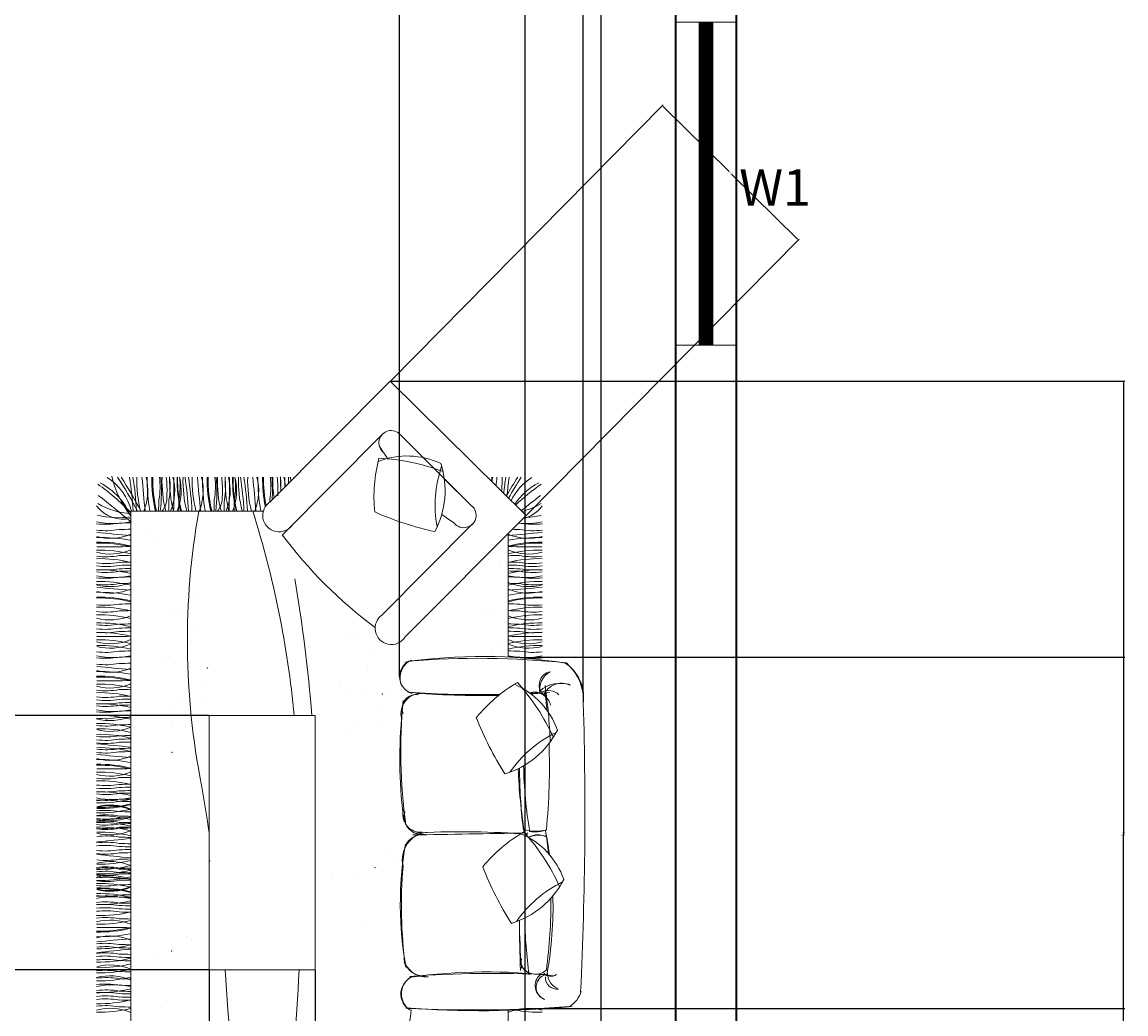
# Model space of a CAD drawing. Units: inches. Extents: x 318 to 927, y -1130 to 13.
# Tile 11 of 17: x 763 to 927, y -587 to -440. Entities that reach past the tile are written whole.
import ezdxf

# ---------------------------------------------------------------- set-up
doc = ezdxf.new("R2010")
doc.units = ezdxf.units.IN
doc.header["$MEASUREMENT"] = 0
for name, color, linetype, lineweight in [('A-ANNO-DIMS', 1, 'Continuous', 18), ('A-ANNO-IDEN', 1, 'Continuous', 13), ('A-FURN-RUGS', 50, 'Continuous', 9), ('A-GLAZ-PATT', 5, 'Continuous', 9), ('wall', 1, 'Continuous', 35), ('win', 5, 'Continuous', 18)]:
    doc.layers.add(name, color=color, linetype=linetype, lineweight=lineweight)
doc.layers.add('furniture', color=50, linetype='Continuous', lineweight=13, transparency=0.8)
doc.styles.get("Standard").update_dxf_attribs({"font": 'arial.ttf'})
doc.dimstyles.get("Standard").update_dxf_attribs({"dimtxt": 0.18, "dimasz": 0.18, "dimexe": 0.18, "dimexo": 0.0625, "dimgap": 0.09, "dimtad": 0, "dimtih": 1, "dimtoh": 1, "dimdec": 1, "dimzin": 0, "dimdsep": 46, "dimlunit": 4, "dimtxsty": 'Standard', "dimcen": 0.09, "dimadec": 0, "dimazin": 0, "dimtfac": 1, "dimtdec": 1, "dimtofl": 0, "dimtmove": 0, "dimatfit": 3, "dimfxl": 1, "dimtolj": 1, "dimtzin": 0, "dimarcsym": 0})

# ---------------------------------------------------------------- blocks, each defined once
blk = doc.blocks.new('WIN-48IN')
for p, q in [((0, 48), (9, 48)), ((3.5, 48), (3.5, 0)), ((5.5, 48), (5.5, 0)), ((0, 0), (9, 0))]:
    blk.add_line(p, q)
blk = doc.blocks.new('*D38')
at = {"layer": 'A-ANNO-DIMS', "color": 0, "lineweight": -2, "transparency": 16777216}
for p, q in [((817.59, -493.51), (926.57, -493.51)), ((926.39, -493.69), (926.39, -560.77)), ((926.39, -628.21), (926.39, -561.13)), ((817.59, -628.39), (926.57, -628.39))]:
    blk.add_line(p, q, dxfattribs=at)
at = {"layer": 'A-ANNO-DIMS', "color": 0, "transparency": 16777216}
for points in [[(926.36, -493.69), (926.42, -493.69), (926.39, -493.51)], [(926.36, -628.21), (926.42, -628.21), (926.39, -628.39)]]:
    blk.add_solid(points, dxfattribs=at)
at = {"layer": 'Defpoints', "color": 0, "transparency": 16777216}
for p in [(817.52, -493.51), (817.52, -628.39), (926.39, -628.39)]:
    blk.add_point(p, dxfattribs=at)
at = {"layer": 'A-ANNO-DIMS', "color": 0, "transparency": 16777216, "insert": (926.39, -560.95), "char_height": 0.18, "attachment_point": 5}
blk.add_mtext('\\A1;11\'-3"', dxfattribs=at)
blk = doc.blocks.new('*D40')
at = {"layer": 'A-ANNO-DIMS', "color": 0, "lineweight": -2, "transparency": 16777216}
for p, q in [((790.65, -580.99), (790.65, -1124.59)), ((806.39, -580.99), (806.39, -1124.59)), ((790.83, -1124.41), (797.99, -1124.41)), ((806.21, -1124.41), (799.05, -1124.41))]:
    blk.add_line(p, q, dxfattribs=at)
at = {"layer": 'A-ANNO-DIMS', "color": 0, "transparency": 16777216}
for points in [[(790.83, -1124.38), (790.83, -1124.44), (790.65, -1124.41)], [(806.21, -1124.38), (806.21, -1124.44), (806.39, -1124.41)]]:
    blk.add_solid(points, dxfattribs=at)
at = {"layer": 'Defpoints', "color": 0, "transparency": 16777216}
for p in [(790.65, -580.93), (806.39, -580.93), (806.39, -1124.41)]:
    blk.add_point(p, dxfattribs=at)
at = {"layer": 'A-ANNO-DIMS', "color": 0, "transparency": 16777216, "insert": (798.52, -1124.41), "char_height": 0.18, "attachment_point": 5}
blk.add_mtext('\\A1;1\'-3 1/2"', dxfattribs=at)
blk = doc.blocks.new('*D41')
at = {"layer": 'A-ANNO-DIMS', "color": 0, "lineweight": -2, "transparency": 16777216}
for p, q in [((790.59, -543.15), (331.21, -543.15)), ((331.39, -543.33), (331.39, -561.86)), ((331.39, -580.75), (331.39, -562.22)), ((790.59, -580.93), (331.21, -580.93))]:
    blk.add_line(p, q, dxfattribs=at)
at = {"layer": 'A-ANNO-DIMS', "color": 0, "transparency": 16777216}
for points in [[(331.36, -543.33), (331.42, -543.33), (331.39, -543.15)], [(331.36, -580.75), (331.42, -580.75), (331.39, -580.93)]]:
    blk.add_solid(points, dxfattribs=at)
at = {"layer": 'Defpoints', "color": 0, "transparency": 16777216}
for p in [(790.65, -543.15), (331.39, -580.93), (790.65, -580.93)]:
    blk.add_point(p, dxfattribs=at)
at = {"layer": 'A-ANNO-DIMS', "color": 0, "transparency": 16777216, "insert": (331.39, -562.04), "char_height": 0.18, "attachment_point": 5}
blk.add_mtext('\\A1;3\'-2"', dxfattribs=at)
blk = doc.blocks.new('*D42')
at = {"layer": 'A-ANNO-DIMS', "color": 0, "lineweight": -2, "transparency": 16777216}
for p, q in [((838.899969, -534.470376), (926.574248, -534.470376)), ((926.394248, -534.650376), (926.394248, -560.388084)), ((926.394248, -586.485792), (926.394248, -560.748084)), ((838.877744, -586.665792), (926.574248, -586.665792))]:
    blk.add_line(p, q, dxfattribs=at)
at = {"layer": 'A-ANNO-DIMS', "color": 0, "transparency": 16777216}
for points in [[(926.364248, -534.650376), (926.424248, -534.650376), (926.394248, -534.470376)], [(926.364248, -586.485792), (926.424248, -586.485792), (926.394248, -586.665792)]]:
    blk.add_solid(points, dxfattribs=at)
at = {"layer": 'Defpoints', "color": 0, "transparency": 16777216}
for p in [(838.837469, -534.470376), (838.815244, -586.665792), (926.394248, -586.665792)]:
    blk.add_point(p, dxfattribs=at)
at = {"layer": 'A-ANNO-DIMS', "color": 0, "transparency": 16777216, "insert": (926.394248, -560.568084), "char_height": 0.18, "attachment_point": 5}
blk.add_mtext('\\A1;4\'-4"', dxfattribs=at)
blk = doc.blocks.new('*D43')
at = {"layer": 'A-ANNO-DIMS', "color": 0, "lineweight": -2, "transparency": 16777216}
for p, q in [((818.92, -537.33), (818.92, -25.23)), ((819.1, -25.41), (832.2, -25.41)), ((845.97, -25.41), (832.87, -25.41)), ((846.15, -539.79), (846.15, -25.23))]:
    blk.add_line(p, q, dxfattribs=at)
at = {"layer": 'A-ANNO-DIMS', "color": 0, "transparency": 16777216}
for points in [[(819.1, -25.38), (819.1, -25.44), (818.92, -25.41)], [(845.97, -25.38), (845.97, -25.44), (846.15, -25.41)]]:
    blk.add_solid(points, dxfattribs=at)
at = {"layer": 'Defpoints', "color": 0, "transparency": 16777216}
for p in [(846.15, -25.41), (818.92, -537.39), (846.15, -539.86)]:
    blk.add_point(p, dxfattribs=at)
at = {"layer": 'A-ANNO-DIMS', "color": 0, "transparency": 16777216, "insert": (832.53, -25.41), "char_height": 0.18, "attachment_point": 5}
blk.add_mtext('\\A1;2\'-3"', dxfattribs=at)
blk = doc.blocks.new('*D44')
at = {"layer": 'A-ANNO-DIMS', "color": 0, "lineweight": -2, "transparency": 16777216}
for p, q in [((817.57, -493.47), (858.05, -452.47)), ((858.05, -452.72), (867.82, -462.37)), ((877.96, -472.38), (868.19, -462.74)), ((837.73, -513.38), (878.22, -472.38))]:
    blk.add_line(p, q, dxfattribs=at)
at = {"layer": 'A-ANNO-DIMS', "color": 0, "transparency": 16777216}
for points in [[(858.07, -452.7), (858.03, -452.74), (857.92, -452.6)], [(877.98, -472.36), (877.94, -472.41), (878.09, -472.51)]]:
    blk.add_solid(points, dxfattribs=at)
at = {"layer": 'Defpoints', "color": 0, "transparency": 16777216}
for p in [(878.09, -472.51), (817.52, -493.51), (837.69, -513.42)]:
    blk.add_point(p, dxfattribs=at)
at = {"layer": 'A-ANNO-DIMS', "color": 0, "transparency": 16777216, "insert": (868.01, -462.55), "char_height": 0.18, "attachment_point": 5}
blk.add_mtext('\\A1;2\'-4 1/2"', dxfattribs=at)
blk = doc.blocks.new('*D53')
at = {"layer": 'A-ANNO-DIMS', "color": 0, "lineweight": -2, "transparency": 16777216}
for p, q in [((837.57, -839.31), (837.57, -25.23)), ((837.75, -25.41), (842.6, -25.41)), ((848.66, -25.41), (843.82, -25.41)), ((848.84, -838.59), (848.84, -25.23))]:
    blk.add_line(p, q, dxfattribs=at)
at = {"layer": 'A-ANNO-DIMS', "color": 0, "transparency": 16777216}
for points in [[(837.75, -25.38), (837.75, -25.44), (837.57, -25.41)], [(848.66, -25.38), (848.66, -25.44), (848.84, -25.41)]]:
    blk.add_solid(points, dxfattribs=at)
at = {"layer": 'Defpoints', "color": 0, "transparency": 16777216}
for p in [(848.84, -25.41), (848.84, -838.66), (837.57, -839.37)]:
    blk.add_point(p, dxfattribs=at)
at = {"layer": 'A-ANNO-DIMS', "color": 0, "transparency": 16777216, "insert": (843.21, -25.41), "char_height": 0.18, "attachment_point": 5}
blk.add_mtext('\\A1;0\'-11 1/2"', dxfattribs=at)

msp = doc.modelspace()

# ---------------------------------------------------------------- hatches: boundary and pattern name
at = {"layer": 'A-GLAZ-PATT'}
h = msp.add_hatch(dxfattribs=at)
h.set_pattern_fill('ANSI31', color=256)
h.paths.add_polyline_path([(865.39, -312.52), (863.39, -312.52), (863.39, -348.52), (865.39, -348.52)])
h.paths.add_polyline_path([(865.39, -440.16), (863.39, -440.16), (863.39, -488.16), (865.39, -488.16)])
h.paths.add_polyline_path([(865.39, -635.51), (863.39, -635.51), (863.39, -683.51), (865.39, -683.51)])
h.paths.add_polyline_path([(865.39, -778.6), (863.39, -778.6), (863.39, -814.6), (865.39, -814.6)])
h.paths.add_polyline_path([(865.39, -834.21), (863.39, -834.21), (863.39, -870.21), (865.39, -870.21)])

# ---------------------------------------------------------------- linework, layer by layer
at = {"layer": 'A-FURN-RUGS'}
for p, q in [((786.52, -509.62), (786.52, -509.62)), ((786.56, -510.1), (786.56, -510.1)), ((794.75, -509.62), (794.75, -509.62)), ((794.79, -510.1), (794.79, -510.1)), ((779, -612.91), (779, -512.79)), ((779, -512.79), (798.69, -512.79)), ((777.42, -514.38), (777.42, -514.38)), ((777.42, -514.38), (777.42, -514.38)), ((777.42, -514.38), (777.42, -514.38)), ((836.61, -514.38), (836.61, -514.38)), ((836.61, -514.38), (836.61, -514.38)), ((836.61, -514.38), (836.61, -514.38)), ((777.71, -515.6), (777.71, -515.6)), ((777.71, -515.6), (777.71, -515.6)), ((777.71, -515.6), (777.71, -515.6)), ((781.73, -515.62), (781.73, -515.62)), ((835.03, -516.09), (835.03, -534.47)), ((836.32, -515.6), (836.32, -515.6)), ((836.32, -515.6), (836.32, -515.6)), ((836.32, -515.6), (836.32, -515.6)), ((782.8, -517.13), (782.8, -517.13)), ((835.56, -518.24), (835.56, -518.24)), ((835.56, -518.24), (835.56, -518.24)), ((832.07, -519.93), (832.07, -519.93)), ((833.84, -520.06), (833.84, -520.06)), ((835.98, -522.53), (835.98, -522.53)), ((835.36, -524.31), (835.36, -524.31)), ((788.26, -525.92), (788.26, -525.92)), ((788.26, -525.92), (788.26, -525.92)), ((784.78, -527.61), (784.78, -527.61)), ((831.36, -527.46), (831.36, -527.46)), ((832.88, -527.58), (832.88, -527.58)), ((779, -528.62), (779, -612.91)), ((786.55, -527.74), (786.55, -527.74)), ((835.06, -528.35), (835.06, -528.35)), ((838, -528.06), (838, -528.06)), ((788.69, -530.21), (788.69, -530.21)), ((814.27, -529.76), (814.27, -529.76)), ((814.27, -529.76), (814.27, -529.76)), ((837.28, -530.85), (837.28, -530.85)), ((788.06, -531.99), (788.06, -531.99)), ((810.79, -531.45), (810.79, -531.45)), ((812.56, -531.58), (812.56, -531.58)), ((814.7, -534.05), (814.7, -534.05)), ((832.56, -534.17), (832.56, -534.17)), ((833.28, -532.67), (833.28, -532.67)), ((837.48, -533.22), (837.48, -533.22)), ((784.07, -535.14), (784.07, -535.14)), ((785.59, -535.26), (785.59, -535.26)), ((790.71, -535.74), (790.71, -535.74)), ((787.77, -536.03), (787.77, -536.03)), ((814.08, -535.83), (814.08, -535.83)), ((789.98, -538.53), (789.98, -538.53)), ((810.08, -538.98), (810.08, -538.98)), ((785.99, -540.35), (785.99, -540.35)), ((811.6, -539.1), (811.6, -539.1)), ((813.78, -539.87), (813.78, -539.87)), ((816.72, -539.59), (816.72, -539.59)), ((785.26, -541.85), (785.26, -541.85)), ((790.19, -540.91), (790.19, -540.91)), ((816, -542.37), (816, -542.37)), ((785.23, -543.92), (785.23, -543.92)), ((812, -544.19), (812, -544.19)), ((816.2, -544.75), (816.2, -544.75)), ((811.28, -545.69), (811.28, -545.69)), ((777.42, -555.75), (777.42, -555.75)), ((777.42, -555.86), (777.42, -555.86)), ((777.42, -559.27), (777.42, -559.27)), ((817.37, -563.55), (817.37, -563.55)), ((817.37, -563.55), (817.37, -563.55)), ((815.49, -565.31), (815.49, -565.31)), ((818.2, -564.09), (818.2, -564.09)), ((818.2, -564.09), (818.2, -564.09)), ((777.42, -566.43), (777.42, -566.43)), ((809.01, -566.45), (809.01, -566.45)), ((812.75, -566.4), (812.75, -566.4)), ((777.42, -569.84), (777.42, -569.84)), ((777.42, -569.95), (777.42, -569.95)), ((813.75, -573.98), (813.75, -573.98)), ((787.23, -575.93), (787.23, -575.93)), ((787.23, -575.93), (787.23, -575.93)), ((788.05, -576.48), (788.05, -576.48)), ((788.05, -576.48), (788.05, -576.48)), ((785.34, -577.7), (785.34, -577.7)), ((778.87, -578.84), (778.87, -578.84)), ((782.6, -578.78), (782.6, -578.78)), ((783.6, -586.37), (783.6, -586.37)), ((835.03, -586.93), (835.03, -589.47))]:
    msp.add_line(p, q, dxfattribs=at)
for centre, radius, start, end in [((771.07, -514.79), 8.28, 13.9935, 57.7288), ((790.74, -504.28), 14.92, 192.9523, 218.0769), ((729.8, -538.65), 56.46, 27.2669, 33.1781), ((730.31, -538.64), 56.46, 27.2669, 33.1781), ((724.61, -515.98), 54.84, 3.3644, 8.6229), ((725.12, -515.97), 54.84, 3.3644, 8.6229), ((799.08, -508.19), 19.18, 178.6331, 193.8573), ((557.89, -530.4), 223.93, 4.5146, 5.8017), ((773.68, -509.76), 7.87, 337.3098, 14.8613), ((806.9, -508.17), 25.47, 179.0195, 190.4039), ((801.3, -508.2), 19.18, 178.6331, 193.8573), ((801.45, -508.2), 19.18, 178.6331, 193.8573), ((771.97, -509.1), 11.39, 349.9349, 6.8829), ((757.66, -509.77), 25.91, 353.3702, 4.5064), ((802.82, -508.19), 19.18, 178.6331, 193.8573), ((766.64, -509.72), 17.75, 357.4435, 6.4413), ((773.46, -509.1), 11.39, 349.9349, 6.8829), ((803.95, -508.18), 19.18, 178.6331, 193.8573), ((777.66, -509.75), 7.87, 337.3098, 14.8613), ((621.19, -508.91), 164.23, 358.628, 0.3934), ((778.63, -509.76), 7.87, 337.3098, 14.8613), ((805.08, -508.2), 19.18, 178.6331, 193.8573), ((805.14, -508.19), 19.18, 178.6331, 193.8573), ((774.95, -509.11), 11.39, 349.9349, 6.8829), ((805.94, -508.2), 19.18, 178.6331, 193.8573), ((732.84, -515.98), 54.84, 3.3644, 8.6229), ((733.35, -515.97), 54.84, 3.3644, 8.6229), ((807.31, -508.19), 19.18, 178.6331, 193.8573), ((566.11, -530.4), 223.93, 4.5146, 5.8017), ((781.9, -509.76), 7.87, 337.3098, 14.8613), ((815.12, -508.17), 25.47, 179.0195, 190.4039), ((809.53, -508.2), 19.18, 178.6331, 193.8573), ((809.67, -508.2), 19.18, 178.6331, 193.8573), ((780.19, -509.1), 11.39, 349.9349, 6.8829), ((765.88, -509.77), 25.91, 353.3702, 4.5064), ((811.04, -508.19), 19.18, 178.6331, 193.8573), ((774.87, -509.72), 17.75, 357.4435, 6.4413), ((781.69, -509.1), 11.39, 349.9349, 6.8829), ((812.18, -508.18), 19.18, 178.6331, 193.8573), ((785.89, -509.75), 7.87, 337.3098, 14.8613), ((629.42, -508.91), 164.23, 358.628, 0.3934), ((786.85, -509.76), 7.87, 337.3098, 14.8613), ((813.3, -508.2), 19.18, 178.6331, 193.8573), ((813.37, -508.19), 19.18, 178.6331, 193.8573), ((783.17, -509.11), 11.39, 349.9349, 6.8829), ((814.16, -508.2), 19.18, 178.6331, 193.8573), ((741.07, -515.98), 54.84, 3.3644, 8.6229), ((741.58, -515.97), 54.84, 3.3644, 8.6229), ((815.54, -508.19), 19.18, 178.6331, 193.8573), ((574.34, -530.4), 223.93, 4.5146, 5.8017), ((790.13, -509.76), 7.87, 337.3098, 14.8613), ((823.36, -508.17), 25.47, 179.0195, 190.4039), ((817.76, -508.2), 19.18, 178.6331, 191.8302), ((817.9, -508.2), 19.18, 178.6331, 191.3519), ((788.42, -509.1), 11.39, 349.9349, 6.8829), ((774.12, -509.77), 25.91, 356.9677, 4.5064), ((819.27, -508.19), 19.18, 178.6331, 187.9798), ((783.1, -509.72), 17.75, 357.4435, 6.4413), ((820.41, -508.18), 19.18, 178.6331, 184.9238), ((789.92, -509.1), 11.39, 356.2453, 6.8829), ((794.12, -509.75), 7.87, 4.2757, 14.8613), ((637.65, -508.91), 164.23, 359.8849, 0.3934), ((821.6, -508.19), 19.18, 178.6331, 181.5238), ((795.08, -509.76), 7.87, 10.6592, 14.8613), ((791.41, -509.11), 11.39, 3.8173, 6.8829), ((822.39, -508.2), 19.18, 178.6331, 179.1046), ((807.13, -508.17), 25.47, 359.4753, 0.9805), ((840.36, -509.76), 7.87, 165.1387, 170.0752), ((1056.15, -530.4), 223.93, 174.1983, 174.5236), ((814.95, -508.19), 19.18, 355.0538, 1.3669), ((888.91, -515.97), 54.84, 171.3771, 173.9203), ((883.72, -538.64), 56.46, 146.8219, 150.1356), ((889.42, -515.98), 54.84, 171.3771, 174.3888), ((884.23, -538.65), 56.46, 146.8219, 150.5026), ((842.96, -514.79), 8.28, 122.2712, 154.6274), ((754.54, -536.39), 33.84, 43.716, 54.6847), ((770.01, -517.21), 9.7, 22.1181, 62.6967), ((844.02, -517.21), 9.7, 117.3033, 145.7016), ((859.49, -536.39), 33.84, 125.3153, 133.6457), ((679.49, -633.67), 155.39, 50.1568, 52.4559), ((910.14, -515.1), 127.02, 178.1891, 178.9775), ((780.95, -510.71), 3.43, 321.6564, 3.1744), ((911.64, -515.1), 127.02, 178.1891, 178.9775), ((913.12, -515.11), 127.02, 178.1891, 178.9775), ((918.36, -515.1), 127.02, 178.1891, 178.9775), ((789.17, -510.71), 3.43, 321.6564, 3.1744), ((919.86, -515.1), 127.02, 178.1891, 178.9775), ((921.35, -515.11), 127.02, 178.1891, 178.9775), ((926.6, -515.1), 127.02, 178.1891, 178.3576), ((934.54, -633.67), 155.39, 127.5441, 128.8901), ((777.91, -509.12), 4.9, 215.9057, 282.8054), ((779.85, -501.71), 11.5, 240.135, 265.7243), ((897.54, -532.05), 110.13, 169.9275, 191.2246), ((656.23, -557.16), 147.71, 5.4421, 17.4799), ((834.18, -501.71), 11.5, 284.6792, 299.865), ((836.12, -509.12), 4.9, 282.9777, 324.0943), ((776.42, -501.87), 12.76, 258.7545, 281.5888), ((777.27, -499.93), 13.84, 256.7215, 277.1491), ((837.61, -501.87), 12.76, 265.1756, 281.2455), ((836.76, -499.93), 13.84, 272.5322, 283.2785), ((775.3, -503.36), 11.39, 263.1171, 280.0651), ((775.29, -504.31), 11.39, 263.1171, 280.0651), ((796.6, -293.17), 223.93, 264.1983, 265.4854), ((781.3, -642.48), 127.02, 91.0225, 91.8109), ((781.3, -641.53), 127.02, 91.0225, 91.8109), ((817.43, -293.17), 223.93, 274.5146, 275.8017), ((832.73, -642.48), 127.02, 88.1891, 88.6709), ((838.74, -503.36), 11.39, 259.9349, 276.8829), ((838.74, -504.31), 11.39, 259.9349, 276.8829), ((774.37, -542.18), 25.47, 79.5961, 90.9805), ((774.4, -536.59), 19.18, 76.1427, 91.3669), ((774.4, -536.73), 19.18, 76.1427, 91.3669), ((775.97, -508.96), 7.87, 255.1387, 292.6902), ((838.07, -508.96), 7.87, 247.3098, 284.8613), ((839.63, -536.59), 19.18, 88.6331, 103.8573), ((839.63, -536.73), 19.18, 88.6331, 103.8573), ((839.66, -542.18), 25.47, 89.0195, 100.4039), ((775.96, -511.3), 7.87, 255.1387, 292.6902), ((774.4, -537.76), 19.18, 76.1427, 91.3669), ((775.3, -508.18), 11.39, 263.1171, 280.0651), ((775.11, -353.87), 164.23, 269.6066, 271.372), ((781.31, -646.35), 127.02, 91.0225, 91.8109), ((838.92, -353.87), 164.23, 268.628, 270.3934), ((832.72, -646.35), 127.02, 88.1891, 88.9775), ((838.07, -511.3), 7.87, 247.3098, 284.8613), ((839.63, -537.76), 19.18, 88.6331, 103.8573), ((838.73, -508.18), 11.39, 259.9349, 276.8829), ((774.4, -539.03), 19.18, 76.1427, 91.3669), ((775.3, -509.18), 11.39, 263.1171, 280.0651), ((775.3, -509.63), 11.39, 263.1171, 280.0651), ((781.31, -647.36), 127.02, 91.0225, 91.8109), ((781.3, -647.81), 127.02, 91.0225, 91.8109), ((832.73, -647.36), 127.02, 88.1891, 88.9775), ((832.73, -647.81), 127.02, 88.1891, 88.9775), ((839.63, -539.03), 19.18, 88.6331, 103.8573), ((838.73, -509.18), 11.39, 259.9349, 276.8829), ((838.73, -509.63), 11.39, 259.9349, 276.8829), ((775.3, -510.14), 11.39, 263.1171, 280.0651), ((774.39, -540.68), 19.18, 76.1427, 91.3669), ((775.3, -510.51), 11.39, 263.1171, 280.0651), ((775.3, -511.38), 11.39, 263.1171, 280.0651), ((776.42, -509.9), 12.76, 258.7545, 281.5888), ((781.3, -648.31), 127.02, 91.0225, 91.8109), ((781.3, -648.68), 127.02, 91.0225, 91.8109), ((781.3, -649.56), 127.02, 91.0225, 91.8109), ((832.73, -648.31), 127.02, 88.1891, 88.9775), ((832.73, -648.68), 127.02, 88.1891, 88.9775), ((832.73, -649.56), 127.02, 88.1891, 88.9775), ((839.64, -540.68), 19.18, 88.6331, 103.8573), ((837.61, -509.9), 12.76, 258.4112, 281.2455), ((838.73, -510.14), 11.39, 259.9349, 276.8829), ((838.73, -510.51), 11.39, 259.9349, 276.8829), ((838.74, -511.38), 11.39, 259.9349, 276.8829), ((774.39, -542.42), 19.18, 76.1427, 91.3669), ((775.95, -516.13), 7.87, 255.1387, 292.6902), ((775.29, -512.34), 11.39, 263.1171, 280.0651), ((796.6, -301.31), 223.93, 264.1983, 265.4854), ((781.3, -650.51), 127.02, 91.0225, 91.8109), ((577.78, -561.59), 228.87, 4.6196, 9.7513), ((832.73, -650.51), 127.02, 88.1891, 88.9775), ((839.64, -542.42), 19.18, 88.6331, 103.8573), ((838.08, -516.13), 7.87, 247.3098, 284.8613), ((817.43, -301.31), 223.93, 274.5146, 275.8017), ((838.74, -512.34), 11.39, 259.9349, 276.8829), ((774.37, -550.32), 25.47, 79.5961, 90.9805), ((774.4, -544.73), 19.18, 76.1427, 91.3669), ((774.4, -544.87), 19.18, 76.1427, 91.3669), ((775.97, -517.1), 7.87, 255.1387, 292.6902), ((838.07, -517.1), 7.87, 247.3098, 284.8613), ((839.63, -544.73), 19.18, 88.6331, 103.8573), ((839.63, -544.87), 19.18, 88.6331, 103.8573), ((839.66, -550.32), 25.47, 89.0195, 100.4039), ((775.3, -515.39), 11.39, 263.1171, 280.0651), ((774.4, -546.24), 19.18, 76.1427, 91.3669), ((775.3, -516.4), 11.39, 263.1171, 280.0651), ((781.31, -653.56), 127.02, 91.0225, 91.8109), ((781.31, -654.57), 127.02, 91.0225, 91.8109), ((832.72, -653.56), 127.02, 88.1891, 88.9775), ((832.73, -654.57), 127.02, 88.1891, 88.9775), ((839.63, -546.24), 19.18, 88.6331, 103.8573), ((838.73, -515.39), 11.39, 259.9349, 276.8829), ((838.73, -516.4), 11.39, 259.9349, 276.8829), ((774.39, -547.37), 19.18, 76.1427, 91.3669), ((775.95, -521.08), 7.87, 255.1387, 292.6902), ((839.64, -547.37), 19.18, 88.6331, 103.8573), ((838.08, -521.08), 7.87, 247.3098, 284.8613), ((774.39, -548.57), 19.18, 76.1427, 91.3669), ((775.3, -519.46), 11.39, 263.1171, 280.0651), ((774.39, -550), 19.18, 76.1427, 91.3669), ((775.31, -518.37), 11.39, 263.1171, 280.0651), ((775.3, -518.96), 11.39, 263.1171, 280.0651), ((781.3, -657.13), 127.02, 91.0225, 91.8109), ((781.3, -657.63), 127.02, 91.0225, 91.8109), ((781.31, -656.54), 127.02, 91.0225, 91.8109), ((832.72, -656.54), 127.02, 88.1891, 88.9775), ((832.73, -657.13), 127.02, 88.1891, 88.9775), ((832.73, -657.63), 127.02, 88.1891, 88.9775), ((839.64, -550), 19.18, 88.6331, 103.8573), ((839.64, -548.57), 19.18, 88.6331, 103.8573), ((838.72, -518.37), 11.39, 259.9349, 276.8829), ((838.73, -518.96), 11.39, 259.9349, 276.8829), ((838.73, -519.46), 11.39, 259.9349, 276.8829), ((775.96, -524.62), 7.87, 255.1387, 292.6902), ((774.4, -551.07), 19.18, 76.1427, 91.3669), ((775.97, -525.28), 7.87, 255.1387, 292.6902), ((775.11, -367.19), 164.23, 269.6066, 271.372), ((838.92, -367.19), 164.23, 268.628, 270.3934), ((838.06, -525.28), 7.87, 247.3098, 284.8613), ((838.07, -524.62), 7.87, 247.3098, 284.8613), ((839.63, -551.07), 19.18, 88.6331, 103.8573), ((775.3, -522.38), 11.39, 263.1171, 280.0651), ((774.41, -551.93), 19.18, 76.1427, 91.3669), ((781.3, -660.55), 127.02, 91.0225, 91.8109), ((832.73, -660.55), 127.02, 88.1891, 88.9775), ((839.62, -551.93), 19.18, 88.6331, 103.8573), ((838.73, -522.38), 11.39, 259.9349, 276.8829), ((775.3, -523.26), 11.39, 263.1171, 280.0651), ((775.29, -524.21), 11.39, 263.1171, 280.0651), ((776.42, -521.77), 12.76, 258.7545, 281.5888), ((781.3, -662.38), 127.02, 91.0225, 91.8109), ((781.3, -661.43), 127.02, 91.0225, 91.8109), ((832.73, -661.43), 127.02, 88.1891, 88.9775), ((837.61, -521.77), 12.76, 258.4112, 281.2455), ((838.74, -523.26), 11.39, 259.9349, 276.8829), ((774.37, -562.08), 25.47, 79.5961, 90.9805), ((774.4, -556.49), 19.18, 76.1427, 91.3669), ((774.4, -556.63), 19.18, 76.1427, 91.3669), ((775.97, -528.86), 7.87, 255.1387, 292.6902), ((796.6, -313.07), 223.93, 264.1983, 265.4854), ((775.96, -531.2), 7.87, 255.1387, 292.6902), ((774.4, -557.66), 19.18, 76.1427, 91.3669), ((775.11, -373.77), 164.23, 269.6066, 271.372), ((775.3, -528.08), 11.39, 263.1171, 280.0651), ((774.4, -558.93), 19.18, 76.1427, 91.3669), ((775.3, -529.08), 11.39, 263.1171, 280.0651), ((781.31, -666.25), 127.02, 91.0225, 91.8109), ((781.31, -667.25), 127.02, 91.0225, 91.8109), ((781.3, -667.71), 127.02, 91.0225, 91.8109), ((775.3, -530.04), 11.39, 263.1171, 280.0651), ((774.39, -560.58), 19.18, 76.1427, 91.3669), ((775.3, -530.41), 11.39, 263.1171, 280.0651), ((775.3, -529.53), 11.39, 263.1171, 280.0651), ((776.42, -529.8), 12.76, 258.7545, 281.5888), ((781.3, -668.21), 127.02, 91.0225, 91.8109), ((781.3, -668.58), 127.02, 91.0225, 91.8109), ((775.3, -531.28), 11.39, 263.1171, 280.0651), ((774.39, -562.32), 19.18, 76.1427, 91.3669), ((775.95, -536.03), 7.87, 255.1387, 292.6902), ((775.29, -532.23), 11.39, 263.1171, 280.0651), ((781.3, -670.41), 127.02, 91.0225, 91.8109), ((781.3, -669.45), 127.02, 91.0225, 91.8109), ((774.39, -563.51), 19.18, 76.1427, 91.3669), ((775.31, -533.32), 11.39, 263.1171, 280.0651), ((775.97, -537.63), 7.87, 255.1387, 292.6902), ((774.41, -564.28), 19.18, 76.1427, 91.3669), ((781.31, -671.49), 127.02, 91.0225, 91.8109), ((775.29, -535.91), 11.39, 263.1171, 280.0651), ((775.31, -535.45), 11.39, 263.1171, 280.0651), ((774.4, -565.12), 19.18, 76.1427, 91.3669), ((775.31, -534.94), 11.39, 263.1171, 280.0651), ((781.3, -674.08), 127.02, 91.0225, 91.8109), ((781.31, -673.12), 127.02, 91.0225, 91.8109), ((781.31, -673.62), 127.02, 91.0225, 91.8109), ((774.41, -567.1), 19.18, 76.1427, 91.3669), ((775.31, -537.33), 11.39, 263.1171, 280.0651), ((734.62, -971.38), 425.85, 84.0165, 84.6992), ((775.32, -536.84), 11.39, 263.1171, 280.0651), ((781.32, -675.5), 127.02, 91.0225, 91.8109), ((781.33, -675.01), 127.02, 91.0225, 91.8109), ((774.37, -575.16), 25.47, 79.5961, 90.9805), ((774.4, -569.57), 19.18, 76.1427, 91.3669), ((774.4, -569.71), 19.18, 76.1427, 91.3669), ((775.97, -541.94), 7.87, 255.1387, 292.6902), ((796.6, -326.15), 223.93, 264.1983, 265.4854), ((775.96, -544.29), 7.87, 255.1387, 292.6902), ((774.4, -570.74), 19.18, 76.1427, 91.3669), ((775.11, -386.85), 164.23, 269.6066, 271.372), ((775.3, -541.16), 11.39, 263.1171, 280.0651), ((774.4, -572.01), 19.18, 76.1427, 91.3669), ((775.3, -542.16), 11.39, 263.1171, 280.0651), ((775.3, -542.62), 11.39, 263.1171, 280.0651), ((781.31, -679.33), 127.02, 91.0225, 91.8109), ((781.31, -680.34), 127.02, 91.0225, 91.8109), ((781.3, -680.79), 127.02, 91.0225, 91.8109), ((578.83, -590.81), 213.96, 8.119, 10.0442), ((775.3, -543.12), 11.39, 263.1171, 280.0651), ((774.39, -573.66), 19.18, 76.1427, 91.3669), ((775.3, -543.49), 11.39, 263.1171, 280.0651), ((776.42, -542.88), 12.76, 258.7545, 281.5888), ((781.3, -681.29), 127.02, 91.0225, 91.8109), ((781.3, -681.66), 127.02, 91.0225, 91.8109), ((775.3, -544.36), 11.39, 263.1171, 280.0651), ((774.39, -538.43), 19.18, 268.6331, 283.8573), ((774.4, -536.93), 19.18, 268.6331, 283.8573), ((775.31, -567.11), 11.39, 79.9349, 96.8829), ((774.41, -537.65), 19.18, 268.6331, 283.8573), ((774.41, -537.77), 19.18, 268.6331, 283.8573), ((775.97, -564.3), 7.87, 67.3098, 104.8613), ((775.97, -564.41), 7.87, 67.3098, 104.8613), ((781.3, -682.54), 127.02, 91.0225, 91.8109), ((781.31, -428.93), 127.02, 268.1891, 268.9775), ((774.39, -577.22), 19.18, 76.1427, 91.3669), ((775.95, -550.93), 7.87, 255.1387, 292.6902), ((775.29, -547.14), 11.39, 263.1171, 280.0651), ((775.31, -568.62), 11.39, 79.9349, 96.8829), ((775.32, -569.29), 11.39, 79.9349, 96.8829), ((734.62, -134.75), 425.85, 275.3008, 275.9835), ((781.3, -685.31), 127.02, 91.0225, 91.8109), ((781.31, -430.45), 127.02, 268.1891, 268.9775), ((781.33, -431.12), 127.02, 268.1891, 268.9775), ((775.29, -570.23), 11.39, 79.9349, 96.8829), ((774.39, -578.88), 19.18, 76.1427, 91.3669), ((775.31, -548.53), 11.39, 263.1171, 280.0651), ((775.31, -548.68), 11.39, 263.1171, 280.0651), ((774.4, -578.2), 19.18, 76.1427, 91.3669), ((775.31, -548.03), 11.39, 263.1171, 280.0651), ((775.97, -553), 7.87, 255.1387, 292.6902), ((781.3, -432.06), 127.02, 268.1891, 268.9775), ((781.31, -686.2), 127.02, 91.0225, 91.8109), ((781.31, -686.7), 127.02, 91.0225, 91.8109), ((781.31, -686.85), 127.02, 91.0225, 91.8109), ((775.29, -573.36), 11.39, 79.9349, 96.8829), ((774.41, -579.65), 19.18, 76.1427, 91.3669), ((775.32, -572.42), 11.39, 79.9349, 96.8829), ((734.62, -137.88), 425.85, 275.3008, 275.9835), ((781.33, -434.25), 127.02, 268.1891, 268.9775), ((775.29, -552.34), 11.39, 263.1171, 280.0651), ((775.31, -573.82), 11.39, 79.9349, 96.8829), ((775.31, -551.88), 11.39, 263.1171, 280.0651), ((781.3, -435.19), 127.02, 268.1891, 268.9775), ((781.3, -690.51), 127.02, 91.0225, 91.8109), ((781.31, -435.65), 127.02, 268.1891, 268.9775), ((781.31, -690.05), 127.02, 91.0225, 91.8109), ((774.41, -546.05), 19.18, 268.6331, 283.8573), ((775.97, -572.7), 7.87, 67.3098, 104.8613), ((734.62, -987.82), 425.85, 84.0165, 84.6992), ((775.32, -553.28), 11.39, 263.1171, 280.0651), ((781.33, -691.45), 127.02, 91.0225, 91.8109), ((774.39, -546.82), 19.18, 268.6331, 283.8573), ((775.29, -555.47), 11.39, 263.1171, 280.0651), ((775.95, -574.77), 7.87, 67.3098, 104.8613), ((775.31, -577.02), 11.39, 79.9349, 96.8829), ((775.31, -577.17), 11.39, 79.9349, 96.8829), ((774.4, -547.5), 19.18, 268.6331, 283.8573), ((775.31, -577.67), 11.39, 79.9349, 96.8829), ((734.62, -990.95), 425.85, 84.0165, 84.6992), ((781.3, -693.64), 127.02, 91.0225, 91.8109), ((781.31, -438.84), 127.02, 268.1891, 268.9775), ((781.31, -439), 127.02, 268.1891, 268.9775), ((781.31, -439.5), 127.02, 268.1891, 268.9775), ((774.39, -548.48), 19.18, 268.6331, 283.8573), ((775.29, -578.56), 11.39, 79.9349, 96.8829), ((774.39, -587.27), 19.18, 76.1427, 91.3669), ((775.31, -557.08), 11.39, 263.1171, 280.0651), ((775.97, -561.29), 7.87, 255.1387, 292.6902), ((775.32, -556.41), 11.39, 263.1171, 280.0651), ((781.3, -440.39), 127.02, 268.1891, 268.9775), ((781.31, -695.25), 127.02, 91.0225, 91.8109), ((781.33, -694.58), 127.02, 91.0225, 91.8109), ((775.3, -581.33), 11.39, 79.9349, 96.8829), ((776.42, -582.82), 12.76, 78.4112, 101.2455), ((775.97, -561.4), 7.87, 255.1387, 292.6902), ((774.41, -587.93), 19.18, 76.1427, 91.3669), ((774.41, -588.04), 19.18, 76.1427, 91.3669), ((774.4, -588.77), 19.18, 76.1427, 91.3669), ((775.31, -558.59), 11.39, 263.1171, 280.0651), ((781.3, -443.16), 127.02, 268.1891, 268.9775), ((781.31, -696.77), 127.02, 91.0225, 91.8109), ((774.39, -552.04), 19.18, 268.6331, 283.8573), ((775.3, -582.21), 11.39, 79.9349, 96.8829), ((775.3, -582.58), 11.39, 79.9349, 96.8829), ((775.3, -583.08), 11.39, 79.9349, 96.8829), ((781.3, -444.04), 127.02, 268.1891, 268.9775), ((781.3, -444.41), 127.02, 268.1891, 268.9775), ((775.3, -583.53), 11.39, 79.9349, 96.8829), ((774.4, -553.69), 19.18, 268.6331, 283.8573), ((775.3, -584.54), 11.39, 79.9349, 96.8829), ((781.3, -444.91), 127.02, 268.1891, 268.9775), ((781.31, -445.36), 127.02, 268.1891, 268.9775), ((781.31, -446.37), 127.02, 268.1891, 268.9775), ((775.96, -581.41), 7.87, 67.3098, 104.8613), ((774.4, -554.96), 19.18, 268.6331, 283.8573), ((774.4, -555.99), 19.18, 268.6331, 283.8573), ((774.4, -556.13), 19.18, 268.6331, 283.8573), ((775.11, -738.85), 164.23, 88.628, 90.3934), ((774.37, -550.53), 25.47, 269.0195, 280.4039), ((775.97, -583.76), 7.87, 67.3098, 104.8613), ((796.6, -799.55), 223.93, 94.5146, 95.8017), ((775.29, -589.79), 11.39, 79.9349, 96.8829), ((775.31, -588.37), 11.39, 79.9349, 96.8829), ((774.41, -558.6), 19.18, 268.6331, 283.8573), ((775.32, -588.86), 11.39, 79.9349, 96.8829), ((734.62, -154.31), 425.85, 275.3008, 275.9835), ((781.32, -450.19), 127.02, 268.1891, 268.9775), ((781.33, -450.69), 127.02, 268.1891, 268.9775), ((775.31, -590.25), 11.39, 79.9349, 96.8829), ((774.4, -560.58), 19.18, 268.6331, 283.8573), ((775.31, -590.76), 11.39, 79.9349, 96.8829), ((774.41, -561.42), 19.18, 268.6331, 283.8573), ((781.3, -451.62), 127.02, 268.1891, 268.9775), ((781.31, -452.08), 127.02, 268.1891, 268.9775), ((781.31, -452.58), 127.02, 268.1891, 268.9775), ((774.39, -562.19), 19.18, 268.6331, 283.8573), ((775.31, -592.38), 11.39, 79.9349, 96.8829), ((775.97, -588.06), 7.87, 67.3098, 104.8613), ((781.31, -454.21), 127.02, 268.1891, 268.9775), ((592.15, -596.67), 201.49, 2.7877, 4.4807), ((-3687.42, -292.9), 4500.67, 356.03178, 356.33069), ((775.95, -589.67), 7.87, 67.3098, 104.8613), ((774.39, -563.38), 19.18, 268.6331, 283.8573), ((775.29, -593.46), 11.39, 79.9349, 96.8829), ((775.3, -594.42), 11.39, 79.9349, 96.8829), ((776.42, -595.9), 12.76, 78.4112, 101.2455), ((781.3, -455.29), 127.02, 268.1891, 268.9775), ((781.3, -456.24), 127.02, 268.1891, 268.9775), ((774.39, -565.12), 19.18, 268.6331, 283.8573), ((775.3, -595.29), 11.39, 79.9349, 96.8829), ((775.3, -595.66), 11.39, 79.9349, 96.8829), ((775.3, -596.17), 11.39, 79.9349, 96.8829), ((781.3, -457.12), 127.02, 268.1891, 268.9775), ((781.3, -457.49), 127.02, 268.1891, 268.9775), ((781.3, -457.99), 127.02, 268.1891, 268.9775), ((775.3, -596.62), 11.39, 79.9349, 96.8829), ((774.4, -566.77), 19.18, 268.6331, 283.8573), ((775.3, -597.62), 11.39, 79.9349, 96.8829), ((781.31, -458.44), 127.02, 268.1891, 268.9775), ((781.31, -459.45), 127.02, 268.1891, 268.9775), ((775.96, -594.5), 7.87, 67.3098, 104.8613), ((774.4, -568.04), 19.18, 268.6331, 283.8573), ((-130.59, -689.06), 929.63, 4.69873, 6.31076), ((1744.62, -689.06), 929.63, 173.68924, 173.93736), ((838.07, -594.5), 7.87, 75.1387, 112.6902), ((839.63, -568.04), 19.18, 259.3731, 271.3669)]:
    msp.add_arc(centre, radius, start, end, dxfattribs=at)
for p in [(837.65, -528.41), (790.36, -536.09), (816.37, -539.93), (785.13, -548.62), (790.71, -564.75), (815.25, -565.74), (785.1, -578.13)]:
    msp.add_point(p, dxfattribs=at)
at = {"layer": 'furniture'}
for p, q in [((817.52, -493.51), (799.75, -511.38)), ((837.69, -513.42), (817.52, -493.51)), ((801.51, -516.3), (816.37, -501.36)), ((829.38, -511.82), (819.03, -501.48)), ((822.39, -504.84), (819.03, -501.48)), ((829.38, -511.82), (825.55, -508)), ((837.69, -513.42), (819.69, -531.53)), ((829.74, -514.7), (816.35, -528.19)), ((790.65, -543.15), (806.39, -543.15)), ((790.65, -580.93), (790.65, -543.15)), ((806.39, -543.15), (806.39, -580.93)), ((806.39, -580.93), (790.65, -580.93))]:
    msp.add_line(p, q, dxfattribs=at)
for centre, radius, start, end in [((817.65, -502.64), 1.81, 40.1092, 229.8908), ((820.03, -516.2), 11.6, 64.4501, 111.7699), ((846.21, -484.81), 35.39, 211.0867, 214.727), ((837.86, -510.71), 22.75, 165.3068, 185.5663), ((814.39, -535.62), 30.72, 69.0815, 87.2768), ((812.67, -509.74), 13, 332.0126, 17.9429), ((841.78, -511.89), 17.59, 160.9005, 190.6513), ((801.02, -513.44), 2.42, 121.4693, 326.9076), ((828.44, -513.41), 1.84, 217.6748, 59.5181), ((834.75, -468.34), 48.67, 246.3371, 257.4176), ((846.21, -484.81), 35.39, 233.5454, 237.1144), ((855.25, -476.38), 66.95, 216.6049, 233.3387), ((817.69, -530.19), 2.41, 123.6335, 326.3665), ((821.52, -537.38), 2.6, 107.7157, 252.8428), ((822.12, -537.6), 3.14, 126.0678, 202.6723), ((831.03, -612.58), 78.21, 80.8079, 98.3514), ((830.53, -661.77), 127.12, 84.0627, 94.6253), ((840.09, -540.47), 6.15, 353.8792, 57.1093), ((838.71, -540.99), 7.52, 8.6549, 48.7104), ((841.62, -538.61), 1.98, 99.2916, 227.6289), ((842.71, -539.32), 3.02, 117.8433, 189.8684), ((847.88, -557.89), 22.75, 120.3068, 140.5663), ((831.4, -549.17), 11.6, 19.4501, 66.7699), ((813.67, -558.92), 30.72, 24.0815, 42.2768), ((842.76, -543), 4.63, 71.2473, 131.1348), ((843, -541.27), 2.93, 64.8715, 156.7247), ((762.42, -550.07), 78.91, 2.2017, 8.3067), ((822.14, -542.88), 3.02, 87.6579, 194.0974), ((821.38, -542.12), 2.09, 80.2617, 201.0115), ((830.44, -399.52), 140.53, 265.8027, 271.3803), ((830.95, -424.57), 115.62, 264.7422, 271.3335), ((838.99, -541.65), 2, 57.7366, 112.2387), ((830.44, -399.52), 140.53, 273.1908, 273.7892), ((839.11, -542.02), 2.23, 10.6216, 109.193), ((830.95, -424.57), 115.62, 273.7101, 275.0653), ((840.98, -541.79), 2.34, 47.7203, 114.4461), ((746.05, -550.8), 95.11, 5.0871, 6.7491), ((283.62, -557.41), 562.8, 357.2697, 1.7875), ((901.3, -548.31), 82.21, 174.8245, 187.7148), ((888.57, -549.59), 69.62, 175.0781, 187.695), ((875.64, -525.74), 48.67, 201.3371, 212.4176), ((830.76, -539.4), 13, 287.0126, 332.9429), ((849.82, -561.5), 17.59, 115.9005, 145.6513), ((746.05, -550.8), 95.11, 354.3639, 2.1219), ((906.18, -549.04), 69.67, 181.6458, 189.5268), ((924.31, -550.2), 87.6, 180.4949, 186.3291), ((902.55, -549.48), 65.24, 181.0061, 189.6001), ((822.03, -557.84), 2.65, 162.9316, 275.1092), ((822.22, -558.17), 2.63, 163.4437, 271.8228), ((810.66, -568.22), 27.87, 15.9625, 17.4638), ((839.11, -553.84), 6.5, 254.0479, 284.2061), ((972.52, -574.44), 135.8, 173.8872, 174.1215), ((839, -555.08), 5.34, 261.5362, 288.3493), ((768.44, -570.99), 72.94, 5.7795, 8.522), ((823.41, -564.56), 4.1, 96.5867, 193.4511), ((822.46, -563.79), 2.99, 84.9234, 155.6374), ((-23893.09, 1385960.41), 1386741.54, 271.02115817, 271.0218453), ((828.07, -682), 121.6, 85.8425, 93.2873), ((848.83, -580.08), 22.75, 120.3068, 140.5663), ((832.35, -571.36), 11.6, 19.4501, 66.7699), ((814.63, -581.11), 30.72, 24.0815, 42.2768), ((828.07, -682), 121.6, 85.3655, 85.4784), ((838.77, -562.02), 1.65, 119.1313, 132.0141), ((917.24, -571.32), 79.78, 172.7245, 172.7726), ((839.4, -563.49), 2.63, 59.8319, 119.468), ((839.59, -564.79), 3.87, 73.3108, 112.6164), ((784.99, -571.52), 56.7, 7.803, 10.4557), ((870.87, -571.22), 51.85, 170.0543, 190.4167), ((888.41, -571.3), 69.23, 175.2072, 187.551), ((876.6, -547.92), 48.67, 201.3371, 212.4176), ((831.71, -561.58), 13, 287.0126, 332.9429), ((850.78, -583.69), 17.59, 115.9005, 145.6513), ((784.99, -571.52), 56.7, 349.9466, 1.5903), ((768.44, -570.99), 72.94, 352.1551, 0.5585), ((917.24, -571.32), 79.78, 181.3731, 187.4472), ((945.88, -572.17), 109.2, 180.7456, 184.456), ((972.52, -574.44), 135.8, 179.6386, 182.7653), ((822.87, -578.58), 3.41, 190.9756, 274.9747), ((822.55, -578.68), 3.15, 199.8228, 272.4985), ((839.11, -579.25), 2.32, 186.1174, 313.1189), ((838.79, -579.69), 1.84, 167.6226, 260.3094), ((833.02, -763.42), 181.97, 87.5073, 93.9592), ((831.83, -662.41), 81.19, 82.9836, 97.989), ((841.25, -583.27), 2.21, 132.3134, 247.6102), ((841.16, -583.49), 1.97, 104.7814, 247.5922), ((841.38, -580.39), 1.49, 224.3938, 303.5856), ((843.5, -581.33), 2.64, 181.184, 247.8216), ((821.89, -584.5), 2.78, 104.6379, 244.3095), ((822.16, -584.5), 2.97, 123.041, 226.0653), ((842.3, -582.04), 1.74, 178.0108, 276.5585), ((842.05, -583), 3.98, 301.8817, 343.9672), ((831.11, -445.04), 141.95, 265.4325, 275.431), ((829.86, -378.53), 208.34, 267.3143, 273.933)]:
    msp.add_arc(centre, radius, start, end, dxfattribs=at)
at = {"layer": 'wall'}
for p, q in [((868.89, -82.91), (868.89, -1042.91)), ((859.89, -433.91), (859.89, -691.91))]:
    msp.add_line(p, q, dxfattribs=at)

# ---------------------------------------------------------------- block references
at = {"layer": 'win'}
msp.add_blockref('WIN-48IN', (859.89, -488.16), dxfattribs=at)

# ---------------------------------------------------------------- texts
at = {"layer": 'A-ANNO-IDEN'}
msp.add_text('W1', height=5.444, dxfattribs=at).set_placement((869.32, -467.45))

# ---------------------------------------------------------------- dimensions: what is measured, and where the dimension line sits
at = {"layer": 'A-ANNO-DIMS'}
for base, p1, p2, picture, middle in [((846.15, -25.41), (818.92, -537.39), (846.15, -539.86), '*D43', (832.53, -25.41)), ((848.84, -25.41), (837.57, -839.37), (848.84, -838.66), '*D53', (843.21, -25.41)), ((806.39, -1124.41), (790.65, -580.93), (806.39, -580.93), '*D40', (798.52, -1124.41))]:
    dim = msp.add_linear_dim(base=base, p1=p1, p2=p2, dimstyle='Standard', override={"dimdec": 1, "dimlfac": 1, "dimrnd": 0, "dimzin": 1, "dimdsep": 46, "dimlunit": 4, "dimfrac": 2}, dxfattribs=at)
    dim.commit()
    dim.dimension.update_dxf_attribs({"geometry": picture, "text_midpoint": middle})
for base, p1, p2, angle, picture, middle in [((878.09, -472.51), (817.52, -493.51), (837.69, -513.42), 315.3615, '*D44', (868.01, -462.55)), ((926.39, -628.39), (817.52, -493.51), (817.52, -628.39), 90, '*D38', (926.39, -560.95)), ((926.39, -586.67), (838.84, -534.47), (838.82, -586.67), 90, '*D42', (926.39, -560.57)), ((331.39, -580.93), (790.65, -543.15), (790.65, -580.93), 90, '*D41', (331.39, -562.04))]:
    dim = msp.add_linear_dim(base=base, p1=p1, p2=p2, angle=angle, dimstyle='Standard', override={"dimdec": 1, "dimlfac": 1, "dimrnd": 0, "dimzin": 1, "dimdsep": 46, "dimlunit": 4, "dimfrac": 2}, dxfattribs=at)
    dim.commit()
    dim.dimension.update_dxf_attribs({"geometry": picture, "text_midpoint": middle})

doc.saveas('drawing.dxf')
